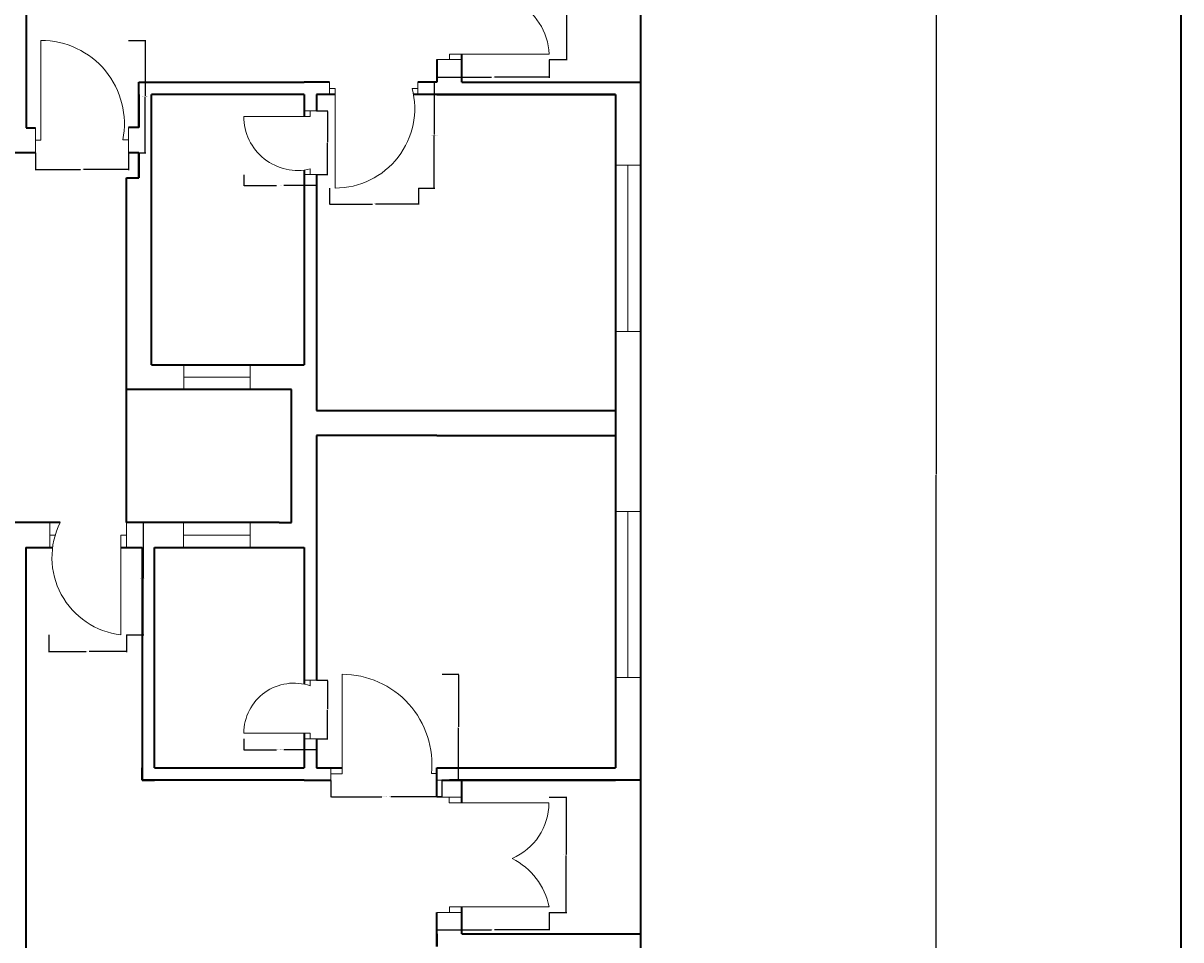
# Model space of a CAD drawing. Units: inches. Extents: x 2250 to 3629, y 982 to 2740.
# Tile 9 of 12: x 3211 to 3629, y 1497 to 1828. Entities that reach past the tile are written whole.
import ezdxf

# ---------------------------------------------------------------- set-up
doc = ezdxf.new("R2010")
doc.units = ezdxf.units.IN
for name, color, linetype, lineweight in [('A-ANNO-DIMS', 2, 'Continuous', 18), ('A-ANNO-TTLB', 7, 'Continuous', 35), ('A-DOOR', 3, 'Continuous', 18), ('A-GLAZ', 4, 'Continuous', 18), ('A-WALL', 7, 'Continuous', 35)]:
    doc.layers.add(name, color=color, linetype=linetype, lineweight=lineweight)
doc.styles.get("Standard").update_dxf_attribs({"font": 'arial.ttf'})
doc.dimstyles.get("Standard").update_dxf_attribs({"dimtxt": 0.18, "dimasz": 0.18, "dimexe": 0.18, "dimexo": 0.0625, "dimgap": 0.09, "dimtad": 0, "dimtih": 1, "dimtoh": 1, "dimdec": 4, "dimzin": 0, "dimdsep": 46, "dimtxsty": 'Standard', "dimcen": 0.09, "dimadec": 0, "dimazin": 0, "dimtfac": 1, "dimtdec": 4, "dimtofl": 0, "dimtmove": 0, "dimatfit": 3, "dimfxl": 1, "dimtolj": 1, "dimtzin": 0, "dimarcsym": 0})

# ---------------------------------------------------------------- blocks, each defined once
blk = doc.blocks.new('DR-36-BED-EAST-N')
for p, q in [((0, 38.25), (0, 33.75)), ((31.87, 33.75), (31.87, 38.25)), ((31.87, 38.25), (31.87, 36)), ((0, 33.75), (0, 36)), ((0, 36), (2, 36)), ((2, 36), (2, 0)), ((31.87, 36), (29.87, 36))]:
    blk.add_line(p, q)
blk.add_arc((2, 28.78), 28.78, 270, 14.5177)
blk = doc.blocks.new('DR-72-DECK-EAST-N')
for p, q in [((9, 42.6), (0, 42.6)), ((0, 42.6), (4.5, 42.6)), ((4.5, 42.6), (4.5, 40.6)), ((4.5, 40.6), (40.5, 40.6)), ((9, 0), (0, 0)), ((0, 0), (4.5, 0)), ((4.5, 0), (4.5, 2)), ((4.5, 2), (40.5, 2))]:
    blk.add_line(p, q)
for centre, radius, start, end in [((18.63, 40.6), 21.87, 295.9981, 0), ((18.59, 1.24), 21.93, 1.9829, 63.9515)]:
    blk.add_arc(centre, radius, start, end)
blk = doc.blocks.new('DR-36-BED-EAST-S')
for p, q in [((4, 2.25), (4, 38.25)), ((0, 4.5), (0, 0)), ((0, 0), (0, 2.25)), ((0, 2.25), (2, 2.25)), ((2, 2.25), (4, 2.25)), ((38.26, 2.37), (36.26, 2.37)), ((40.06, 0), (38.26, 0))]:
    blk.add_line(p, q)
blk.add_arc((4, 5.8), 32.45, 353.93, 90)
blk = doc.blocks.new('DR-72-DECK-EAST-S')
for p, q in [((5.33, 41.58), (0, 41.58)), ((0, 41.58), (4.45, 41.58)), ((9, 41.58), (1.67, 41.58)), ((1.67, 41.58), (5.33, 41.58)), ((4.45, 41.58), (4.45, 39.58)), ((4.45, 39.58), (40.45, 39.58)), ((4.5, 0), (4.5, 2)), ((4.5, 2), (40.5, 2)), ((9, 0), (0, 0)), ((0, 0), (4.5, 0))]:
    blk.add_line(p, q)
for centre, radius, start, end in [((18.64, 39.58), 21.82, 293.079, 0), ((16.02, -2.8), 24.94, 11.0871, 63.4091)]:
    blk.add_arc(centre, radius, start, end)
blk = doc.blocks.new('DR-24-BATH-EAST-S')
for p, q in [((21.75, 21.12), (26.25, 21.12)), ((26.25, 21.12), (24, 21.12)), ((24, 21.12), (24, 19.12)), ((24, 2), (0, 2)), ((24, 0), (24, 2)), ((26.25, 0), (21.75, 0)), ((21.75, 0), (24, 0))]:
    blk.add_line(p, q)
blk.add_arc((18.1, 2), 18.1, 70.988, 180)
blk = doc.blocks.new('DR-36-ENTRY-SE')
for p, q in [((0, 31.5), (0, 40.5)), ((27.72, 40.5), (27.72, 31.5)), ((0, 36), (2, 36)), ((27.72, 36), (25.72, 36)), ((25.72, 36), (25.72, 0)), ((27.72, 31.5), (27.72, 36))]:
    blk.add_line(p, q)
blk.add_arc((28.88, 27.9), 28.08, 153.3297, 263.5366)
blk = doc.blocks.new('DR-24-BATH-EAST-N')
for p, q in [((24, 20.95), (0, 20.95)), ((26.25, 22.95), (21.75, 22.95)), ((21.75, 22.95), (24, 22.95)), ((24, 22.95), (24, 20.95)), ((24, 0), (24, 2)), ((21.75, 0), (26.25, 0)), ((26.25, 0), (24, 0))]:
    blk.add_line(p, q)
blk.add_arc((19.48, 20.95), 19.48, 180, 283.4076)
blk = doc.blocks.new('DR-36-ENTRY-NE')
for p, q in [((2, 4.58), (2, 40.58)), ((0, 9), (0, 0)), ((33.56, 9.15), (33.56, 0.15)), ((0, 4.58), (2, 4.58)), ((33.56, 4.65), (31.56, 4.65))]:
    blk.add_line(p, q)
blk.add_arc((2, 10.45), 30.13, 348.9073, 90)
blk = doc.blocks.new('WIN-24-BATH-NW')
for p, q in [((9, 24), (0, 24)), ((0, 24), (4.5, 24)), ((4.5, 24), (4.5, 0)), ((9, 0), (0, 0)), ((4.5, 0), (9, 0))]:
    blk.add_line(p, q)
blk = doc.blocks.new('WIN-60-BED-EAST-S')
for p, q in [((0, 60), (9, 60)), ((9, 60), (4.5, 60)), ((4.5, 60), (4.5, 0)), ((9, 0), (0, 0)), ((4.5, 0), (9, 0))]:
    blk.add_line(p, q)
blk = doc.blocks.new('*D113')
at = {"layer": 'A-ANNO-DIMS', "color": 0, "lineweight": -2, "transparency": 16777216}
for p, q in [((3354.1, 1806.24), (3359.95, 1806.24)), ((3359.77, 1806.06), (3359.77, 1787.29)), ((3359.77, 1768.17), (3359.77, 1786.93)), ((3354.1, 1767.99), (3359.95, 1767.99))]:
    blk.add_line(p, q, dxfattribs=at)
at = {"layer": 'A-ANNO-DIMS', "color": 0, "transparency": 16777216}
for points in [[(3359.74, 1806.06), (3359.8, 1806.06), (3359.77, 1806.24)], [(3359.74, 1768.17), (3359.8, 1768.17), (3359.77, 1767.99)]]:
    blk.add_solid(points, dxfattribs=at)
at = {"layer": 'Defpoints', "color": 0, "transparency": 16777216}
for p in [(3354.04, 1806.24), (3359.77, 1806.24), (3354.04, 1767.99)]:
    blk.add_point(p, dxfattribs=at)
at = {"layer": 'A-ANNO-DIMS', "color": 0, "transparency": 16777216, "insert": (3359.77, 1787.11), "char_height": 0.18, "attachment_point": 5}
blk.add_mtext('\\A1;BEDROOM DOOR 38 TYP.', dxfattribs=at)
blk = doc.blocks.new('*D114')
at = {"layer": 'A-ANNO-DIMS', "color": 0, "lineweight": -2, "transparency": 16777216}
for p, q in [((3321.94, 1767.92), (3321.94, 1762.07)), ((3354.04, 1767.92), (3354.04, 1762.07)), ((3322.12, 1762.25), (3337.46, 1762.25)), ((3353.86, 1762.25), (3338.52, 1762.25))]:
    blk.add_line(p, q, dxfattribs=at)
at = {"layer": 'A-ANNO-DIMS', "color": 0, "transparency": 16777216}
for points in [[(3322.12, 1762.28), (3322.12, 1762.22), (3321.94, 1762.25)], [(3353.86, 1762.28), (3353.86, 1762.22), (3354.04, 1762.25)]]:
    blk.add_solid(points, dxfattribs=at)
at = {"layer": 'Defpoints', "color": 0, "transparency": 16777216}
for p in [(3321.94, 1767.99), (3354.04, 1767.99), (3354.04, 1762.25)]:
    blk.add_point(p, dxfattribs=at)
at = {"layer": 'A-ANNO-DIMS', "color": 0, "transparency": 16777216, "insert": (3337.99, 1762.25), "char_height": 0.18, "attachment_point": 5}
blk.add_mtext('\\A1;32 TYP.', dxfattribs=at)
blk = doc.blocks.new('*D115')
at = {"layer": 'A-ANNO-DIMS', "color": 0, "lineweight": -2, "transparency": 16777216}
for p, q in [((3401.29, 1856.98), (3407.8, 1856.98)), ((3407.62, 1856.8), (3407.62, 1835.86)), ((3407.62, 1814.56), (3407.62, 1835.5)), ((3401.29, 1814.38), (3407.8, 1814.38))]:
    blk.add_line(p, q, dxfattribs=at)
at = {"layer": 'A-ANNO-DIMS', "color": 0, "transparency": 16777216}
for points in [[(3407.59, 1856.8), (3407.65, 1856.8), (3407.62, 1856.98)], [(3407.59, 1814.56), (3407.65, 1814.56), (3407.62, 1814.38)]]:
    blk.add_solid(points, dxfattribs=at)
at = {"layer": 'Defpoints', "color": 0, "transparency": 16777216}
for p in [(3401.23, 1856.98), (3407.62, 1856.98), (3401.23, 1814.38)]:
    blk.add_point(p, dxfattribs=at)
at = {"layer": 'A-ANNO-DIMS', "color": 0, "transparency": 16777216, "insert": (3407.62, 1835.68), "char_height": 0.18, "attachment_point": 5}
blk.add_mtext('\\A1;DECK DOOR 43 TYP.', dxfattribs=at)
blk = doc.blocks.new('*D116')
at = {"layer": 'A-ANNO-DIMS', "color": 0, "lineweight": -2, "transparency": 16777216}
for p, q in [((3360.73, 1814.32), (3360.73, 1807.81)), ((3401.23, 1814.32), (3401.23, 1807.81)), ((3360.91, 1807.99), (3380.45, 1807.99)), ((3401.05, 1807.99), (3381.51, 1807.99))]:
    blk.add_line(p, q, dxfattribs=at)
at = {"layer": 'A-ANNO-DIMS', "color": 0, "transparency": 16777216}
for points in [[(3360.91, 1808.02), (3360.91, 1807.96), (3360.73, 1807.99)], [(3401.05, 1808.02), (3401.05, 1807.96), (3401.23, 1807.99)]]:
    blk.add_solid(points, dxfattribs=at)
at = {"layer": 'Defpoints', "color": 0, "transparency": 16777216}
for p in [(3360.73, 1814.38), (3401.23, 1814.38), (3401.23, 1807.99)]:
    blk.add_point(p, dxfattribs=at)
at = {"layer": 'A-ANNO-DIMS', "color": 0, "transparency": 16777216, "insert": (3380.98, 1807.99), "char_height": 0.18, "attachment_point": 5}
blk.add_mtext('\\A1;41 TYP.', dxfattribs=at)
blk = doc.blocks.new('*D117')
at = {"layer": 'A-ANNO-DIMS', "color": 0, "lineweight": -2, "transparency": 16777216}
for p, q in [((3322.46, 1554.17), (3322.46, 1548.05)), ((3362.53, 1554.17), (3362.53, 1548.05)), ((3322.64, 1548.23), (3340.87, 1548.23)), ((3362.35, 1548.23), (3344.11, 1548.23))]:
    blk.add_line(p, q, dxfattribs=at)
at = {"layer": 'A-ANNO-DIMS', "color": 0, "transparency": 16777216}
for points in [[(3322.64, 1548.26), (3322.64, 1548.2), (3322.46, 1548.23)], [(3362.35, 1548.26), (3362.35, 1548.2), (3362.53, 1548.23)]]:
    blk.add_solid(points, dxfattribs=at)
at = {"layer": 'Defpoints', "color": 0, "transparency": 16777216}
for p in [(3322.46, 1554.24), (3362.53, 1554.24), (3362.53, 1548.23)]:
    blk.add_point(p, dxfattribs=at)
at = {"layer": 'A-ANNO-DIMS', "color": 0, "transparency": 16777216, "insert": (3342.49, 1548.23), "char_height": 0.18, "attachment_point": 5}
blk.add_mtext('\\A1;BEDROOM DOOR 40 TYP.', dxfattribs=at)
blk = doc.blocks.new('*D118')
at = {"layer": 'A-ANNO-DIMS', "color": 0, "lineweight": -2, "transparency": 16777216}
for p, q in [((3362.59, 1592.49), (3368.71, 1592.49)), ((3368.53, 1592.31), (3368.53, 1573.54)), ((3368.53, 1554.42), (3368.53, 1573.18)), ((3362.59, 1554.24), (3368.71, 1554.24))]:
    blk.add_line(p, q, dxfattribs=at)
at = {"layer": 'A-ANNO-DIMS', "color": 0, "transparency": 16777216}
for points in [[(3368.5, 1592.31), (3368.56, 1592.31), (3368.53, 1592.49)], [(3368.5, 1554.42), (3368.56, 1554.42), (3368.53, 1554.24)]]:
    blk.add_solid(points, dxfattribs=at)
at = {"layer": 'Defpoints', "color": 0, "transparency": 16777216}
for p in [(3362.53, 1592.49), (3368.53, 1592.49), (3362.53, 1554.24)]:
    blk.add_point(p, dxfattribs=at)
at = {"layer": 'A-ANNO-DIMS', "color": 0, "transparency": 16777216, "insert": (3368.53, 1573.36), "char_height": 0.18, "attachment_point": 5}
blk.add_mtext('\\A1;38 TYP.', dxfattribs=at)
blk = doc.blocks.new('*D119')
at = {"layer": 'A-ANNO-DIMS', "color": 0, "lineweight": -2, "transparency": 16777216}
for p, q in [((3401.29, 1548.06), (3407.64, 1548.06)), ((3407.46, 1547.88), (3407.46, 1527.45)), ((3407.46, 1506.66), (3407.46, 1527.09)), ((3401.29, 1506.48), (3407.64, 1506.48))]:
    blk.add_line(p, q, dxfattribs=at)
at = {"layer": 'A-ANNO-DIMS', "color": 0, "transparency": 16777216}
for points in [[(3407.43, 1547.88), (3407.49, 1547.88), (3407.46, 1548.06)], [(3407.43, 1506.66), (3407.49, 1506.66), (3407.46, 1506.48)]]:
    blk.add_solid(points, dxfattribs=at)
at = {"layer": 'Defpoints', "color": 0, "transparency": 16777216}
for p in [(3401.23, 1548.06), (3407.46, 1548.06), (3401.23, 1506.48)]:
    blk.add_point(p, dxfattribs=at)
at = {"layer": 'A-ANNO-DIMS', "color": 0, "transparency": 16777216, "insert": (3407.46, 1527.27), "char_height": 0.18, "attachment_point": 5}
blk.add_mtext('\\A1;DECK DOOR 42 TYP.', dxfattribs=at)
blk = doc.blocks.new('*D120')
at = {"layer": 'A-ANNO-DIMS', "color": 0, "lineweight": -2, "transparency": 16777216}
for p, q in [((3360.73, 1506.42), (3360.73, 1500.06)), ((3401.23, 1506.42), (3401.23, 1500.06)), ((3360.91, 1500.24), (3380.45, 1500.24)), ((3401.05, 1500.24), (3381.51, 1500.24))]:
    blk.add_line(p, q, dxfattribs=at)
at = {"layer": 'A-ANNO-DIMS', "color": 0, "transparency": 16777216}
for points in [[(3360.91, 1500.27), (3360.91, 1500.21), (3360.73, 1500.24)], [(3401.05, 1500.27), (3401.05, 1500.21), (3401.23, 1500.24)]]:
    blk.add_solid(points, dxfattribs=at)
at = {"layer": 'Defpoints', "color": 0, "transparency": 16777216}
for p in [(3360.73, 1506.48), (3401.23, 1506.48), (3401.23, 1500.24)]:
    blk.add_point(p, dxfattribs=at)
at = {"layer": 'A-ANNO-DIMS', "color": 0, "transparency": 16777216, "insert": (3380.98, 1500.24), "char_height": 0.18, "attachment_point": 5}
blk.add_mtext('\\A1;41 TYP.', dxfattribs=at)
blk = doc.blocks.new('*D131')
at = {"layer": 'A-ANNO-DIMS', "color": 0, "lineweight": -2, "transparency": 16777216}
for p, q in [((3290.98, 1569.11), (3290.98, 1565.05)), ((3317.23, 1569.11), (3317.23, 1565.05)), ((3291.16, 1565.23), (3302.8, 1565.23)), ((3317.05, 1565.23), (3305.41, 1565.23))]:
    blk.add_line(p, q, dxfattribs=at)
at = {"layer": 'A-ANNO-DIMS', "color": 0, "transparency": 16777216}
for points in [[(3291.16, 1565.26), (3291.16, 1565.2), (3290.98, 1565.23)], [(3317.05, 1565.26), (3317.05, 1565.2), (3317.23, 1565.23)]]:
    blk.add_solid(points, dxfattribs=at)
at = {"layer": 'Defpoints', "color": 0, "transparency": 16777216}
for p in [(3290.98, 1569.17), (3317.23, 1569.17), (3317.23, 1565.23)]:
    blk.add_point(p, dxfattribs=at)
at = {"layer": 'A-ANNO-DIMS', "color": 0, "transparency": 16777216, "insert": (3304.1, 1565.23), "char_height": 0.18, "attachment_point": 5}
blk.add_mtext('\\A1;BATH DOOR 26 TYP.', dxfattribs=at)
blk = doc.blocks.new('*D132')
at = {"layer": 'A-ANNO-DIMS', "color": 0, "lineweight": -2, "transparency": 16777216}
for p, q in [((3317.29, 1590.29), (3321.34, 1590.29)), ((3321.16, 1590.11), (3321.16, 1579.91)), ((3321.16, 1569.35), (3321.16, 1579.55)), ((3317.29, 1569.17), (3321.34, 1569.17))]:
    blk.add_line(p, q, dxfattribs=at)
at = {"layer": 'A-ANNO-DIMS', "color": 0, "transparency": 16777216}
for points in [[(3321.13, 1590.11), (3321.19, 1590.11), (3321.16, 1590.29)], [(3321.13, 1569.35), (3321.19, 1569.35), (3321.16, 1569.17)]]:
    blk.add_solid(points, dxfattribs=at)
at = {"layer": 'Defpoints', "color": 0, "transparency": 16777216}
for p in [(3317.23, 1590.29), (3321.16, 1590.29), (3317.23, 1569.17)]:
    blk.add_point(p, dxfattribs=at)
at = {"layer": 'A-ANNO-DIMS', "color": 0, "transparency": 16777216, "insert": (3321.16, 1579.73), "char_height": 0.18, "attachment_point": 5}
blk.add_mtext('\\A1;21 TYP.', dxfattribs=at)
blk = doc.blocks.new('*D133')
at = {"layer": 'A-ANNO-DIMS', "color": 0, "lineweight": -2, "transparency": 16777216}
for p, q in [((3248.66, 1647.24), (3254.85, 1647.24)), ((3254.67, 1647.06), (3254.67, 1627.17)), ((3254.67, 1606.92), (3254.67, 1626.8)), ((3248.66, 1606.74), (3254.85, 1606.74))]:
    blk.add_line(p, q, dxfattribs=at)
at = {"layer": 'A-ANNO-DIMS', "color": 0, "transparency": 16777216}
for points in [[(3254.64, 1647.06), (3254.7, 1647.06), (3254.67, 1647.24)], [(3254.64, 1606.92), (3254.7, 1606.92), (3254.67, 1606.74)]]:
    blk.add_solid(points, dxfattribs=at)
at = {"layer": 'Defpoints', "color": 0, "transparency": 16777216}
for p in [(3248.6, 1647.24), (3254.67, 1647.24), (3248.6, 1606.74)]:
    blk.add_point(p, dxfattribs=at)
at = {"layer": 'A-ANNO-DIMS', "color": 0, "transparency": 16777216, "insert": (3254.67, 1626.99), "char_height": 0.18, "attachment_point": 5}
blk.add_mtext('\\A1;ENTRY DOOR 41 TYP.', dxfattribs=at)
blk = doc.blocks.new('*D134')
at = {"layer": 'A-ANNO-DIMS', "color": 0, "lineweight": -2, "transparency": 16777216}
for p, q in [((3220.55, 1606.67), (3220.55, 1600.48)), ((3248.6, 1606.67), (3248.6, 1600.48)), ((3220.73, 1600.66), (3234.04, 1600.66)), ((3248.42, 1600.66), (3235.1, 1600.66))]:
    blk.add_line(p, q, dxfattribs=at)
at = {"layer": 'A-ANNO-DIMS', "color": 0, "transparency": 16777216}
for points in [[(3220.73, 1600.69), (3220.73, 1600.63), (3220.55, 1600.66)], [(3248.42, 1600.69), (3248.42, 1600.63), (3248.6, 1600.66)]]:
    blk.add_solid(points, dxfattribs=at)
at = {"layer": 'Defpoints', "color": 0, "transparency": 16777216}
for p in [(3220.55, 1606.74), (3248.6, 1606.74), (3248.6, 1600.66)]:
    blk.add_point(p, dxfattribs=at)
at = {"layer": 'A-ANNO-DIMS', "color": 0, "transparency": 16777216, "insert": (3234.57, 1600.66), "char_height": 0.18, "attachment_point": 5}
blk.add_mtext('\\A1;28 TYP.', dxfattribs=at)
blk = doc.blocks.new('*D139')
at = {"layer": 'A-ANNO-DIMS', "color": 0, "lineweight": -2, "transparency": 16777216}
for p, q in [((3290.98, 1772.83), (3290.98, 1768.77)), ((3291.16, 1768.95), (3302.8, 1768.95)), ((3317.05, 1768.95), (3305.41, 1768.95)), ((3317.23, 1772.83), (3317.23, 1768.77))]:
    blk.add_line(p, q, dxfattribs=at)
at = {"layer": 'A-ANNO-DIMS', "color": 0, "transparency": 16777216}
for points in [[(3291.16, 1768.98), (3291.16, 1768.92), (3290.98, 1768.95)], [(3317.05, 1768.98), (3317.05, 1768.92), (3317.23, 1768.95)]]:
    blk.add_solid(points, dxfattribs=at)
at = {"layer": 'Defpoints', "color": 0, "transparency": 16777216}
for p in [(3290.98, 1772.89), (3317.23, 1772.89), (3317.23, 1768.95)]:
    blk.add_point(p, dxfattribs=at)
at = {"layer": 'A-ANNO-DIMS', "color": 0, "transparency": 16777216, "insert": (3304.1, 1768.95), "char_height": 0.18, "attachment_point": 5}
blk.add_mtext('\\A1;BATH DOOR 26 TYP.', dxfattribs=at)
blk = doc.blocks.new('*D140')
at = {"layer": 'A-ANNO-DIMS', "color": 0, "lineweight": -2, "transparency": 16777216}
for p, q in [((3317.29, 1795.84), (3321.34, 1795.84)), ((3321.16, 1795.66), (3321.16, 1784.55)), ((3321.16, 1773.07), (3321.16, 1784.18)), ((3317.29, 1772.89), (3321.34, 1772.89))]:
    blk.add_line(p, q, dxfattribs=at)
at = {"layer": 'A-ANNO-DIMS', "color": 0, "transparency": 16777216}
for points in [[(3321.13, 1795.66), (3321.19, 1795.66), (3321.16, 1795.84)], [(3321.13, 1773.07), (3321.19, 1773.07), (3321.16, 1772.89)]]:
    blk.add_solid(points, dxfattribs=at)
at = {"layer": 'Defpoints', "color": 0, "transparency": 16777216}
for p in [(3317.23, 1795.84), (3321.16, 1795.84), (3317.23, 1772.89)]:
    blk.add_point(p, dxfattribs=at)
at = {"layer": 'A-ANNO-DIMS', "color": 0, "transparency": 16777216, "insert": (3321.16, 1784.37), "char_height": 0.18, "attachment_point": 5}
blk.add_mtext('\\A1;23 TYP.', dxfattribs=at)
blk = doc.blocks.new('*D145')
at = {"layer": 'A-ANNO-DIMS', "color": 0, "lineweight": -2, "transparency": 16777216}
for p, q in [((3249.35, 1821.31), (3255.55, 1821.31)), ((3255.37, 1821.13), (3255.37, 1801.21)), ((3255.37, 1780.92), (3255.37, 1800.84)), ((3249.35, 1780.74), (3255.55, 1780.74))]:
    blk.add_line(p, q, dxfattribs=at)
at = {"layer": 'A-ANNO-DIMS', "color": 0, "transparency": 16777216}
for points in [[(3255.34, 1821.13), (3255.4, 1821.13), (3255.37, 1821.31)], [(3255.34, 1780.92), (3255.4, 1780.92), (3255.37, 1780.74)]]:
    blk.add_solid(points, dxfattribs=at)
at = {"layer": 'Defpoints', "color": 0, "transparency": 16777216}
for p in [(3249.29, 1821.31), (3255.37, 1821.31), (3249.29, 1780.74)]:
    blk.add_point(p, dxfattribs=at)
at = {"layer": 'A-ANNO-DIMS', "color": 0, "transparency": 16777216, "insert": (3255.37, 1801.02), "char_height": 0.18, "attachment_point": 5}
blk.add_mtext('\\A1;ENTRY DOOR 41 TYP.', dxfattribs=at)
blk = doc.blocks.new('*D146')
at = {"layer": 'A-ANNO-DIMS', "color": 0, "lineweight": -2, "transparency": 16777216}
for p, q in [((3215.72, 1780.67), (3215.72, 1774.47)), ((3249.29, 1780.67), (3249.29, 1774.47)), ((3215.9, 1774.65), (3231.97, 1774.65)), ((3249.11, 1774.65), (3233.03, 1774.65))]:
    blk.add_line(p, q, dxfattribs=at)
at = {"layer": 'A-ANNO-DIMS', "color": 0, "transparency": 16777216}
for points in [[(3215.9, 1774.68), (3215.9, 1774.62), (3215.72, 1774.65)], [(3249.11, 1774.68), (3249.11, 1774.62), (3249.29, 1774.65)]]:
    blk.add_solid(points, dxfattribs=at)
at = {"layer": 'Defpoints', "color": 0, "transparency": 16777216}
for p in [(3215.72, 1780.74), (3249.29, 1780.74), (3249.29, 1774.65)]:
    blk.add_point(p, dxfattribs=at)
at = {"layer": 'A-ANNO-DIMS', "color": 0, "transparency": 16777216, "insert": (3232.5, 1774.65), "char_height": 0.18, "attachment_point": 5}
blk.add_mtext('\\A1;34 TYP.', dxfattribs=at)
blk = doc.blocks.new('*D172')
at = {"layer": 'A-ANNO-DIMS', "color": 0, "lineweight": -2, "transparency": 16777216}
for p, q in [((3433.02, 2070.24), (3541.21, 2070.24)), ((3541.03, 2070.06), (3541.03, 1664.67)), ((3541.03, 1258.92), (3541.03, 1664.3)), ((3059.29, 1258.74), (3541.21, 1258.74))]:
    blk.add_line(p, q, dxfattribs=at)
at = {"layer": 'A-ANNO-DIMS', "color": 0, "transparency": 16777216}
for points in [[(3541, 2070.06), (3541.06, 2070.06), (3541.03, 2070.24)], [(3541, 1258.92), (3541.06, 1258.92), (3541.03, 1258.74)]]:
    blk.add_solid(points, dxfattribs=at)
at = {"layer": 'Defpoints', "color": 0, "transparency": 16777216}
for p in [(3432.96, 2070.24), (3541.03, 2070.24), (3059.23, 1258.74)]:
    blk.add_point(p, dxfattribs=at)
at = {"layer": 'A-ANNO-DIMS', "color": 0, "transparency": 16777216, "insert": (3541.03, 1664.49), "char_height": 0.18, "attachment_point": 5}
blk.add_mtext('\\A1;811.5', dxfattribs=at)

msp = doc.modelspace()

# ---------------------------------------------------------------- linework, layer by layer
at = {"layer": 'A-ANNO-TTLB'}
msp.add_lwpolyline([(2249.6849, 2739.593), (3629.4532, 2739.593), (3629.4532, 982.3108), (2249.6849, 982.3108)], close=True, dxfattribs=at)
at = {"layer": 'A-WALL'}
for p, q in [((3434.2267, 2029.7354), (3434.2267, 1276.7354)), ((3212.321, 1926.2354), (3212.321, 1789.7354)), ((3369.7267, 1806.2354), (3369.7267, 1816.3801)), ((3360.7267, 1814.3801), (3360.7267, 1806.2354)), ((3253.0965, 1806.2354), (3312.7267, 1806.2354)), ((3253.0965, 1789.8862), (3253.0965, 1806.2354)), ((3321.9387, 1806.2354), (3312.7267, 1806.2354)), ((3360.7267, 1806.2354), (3353.804, 1806.2354)), ((3369.7267, 1806.2354), (3434.2267, 1806.2354)), ((3253.0965, 1801.7354), (3253.0965, 1789.8862)), ((3312.7267, 1801.7354), (3257.5965, 1801.7354)), ((3257.5965, 1704.2354), (3257.5965, 1801.7354)), ((3312.7267, 1801.7354), (3312.7267, 1793.8422)), ((3323.9387, 1801.7354), (3317.2267, 1801.7354)), ((3317.2267, 1801.7354), (3317.2267, 1795.8422)), ((3425.2267, 1801.7354), (3352.2915, 1801.7354)), ((3360.7267, 1801.7354), (3425.2267, 1801.7354)), ((3360.7267, 1801.7354), (3369.7267, 1801.7354)), ((3425.2267, 1801.7354), (3425.2267, 1558.7354)), ((3253.0965, 1789.8862), (3249.2854, 1789.8862)), ((3212.321, 1789.7354), (3215.7202, 1789.7354)), ((3212.321, 1780.7354), (3203.2267, 1780.7354)), ((3215.7202, 1780.7354), (3212.321, 1780.7354)), ((3249.2854, 1780.8862), (3253.0965, 1780.8862)), ((3253.0965, 1780.8862), (3253.0965, 1771.6808)), ((3253.0965, 1771.6808), (3253.0965, 1780.8862)), ((3312.7267, 1774.4922), (3312.7267, 1704.2354)), ((3248.5965, 1704.2354), (3248.5965, 1771.6808)), ((3248.5965, 1771.6808), (3253.0965, 1771.6808)), ((3317.2267, 1772.8908), (3317.2267, 1687.7354)), ((3248.5965, 1647.2354), (3248.5965, 1704.2354)), ((3257.5965, 1704.2354), (3312.7267, 1704.2354)), ((3308.2267, 1695.2354), (3248.5965, 1695.2354)), ((3308.2267, 1647.2354), (3308.2267, 1695.2354)), ((3317.2267, 1687.7354), (3360.7267, 1687.7354)), ((3360.7267, 1687.7354), (3425.2267, 1687.7354)), ((3360.7267, 1678.7354), (3317.2267, 1678.7354)), ((3317.2267, 1678.7354), (3317.2267, 1590.2852)), ((3360.7267, 1678.7354), (3425.2267, 1678.7354)), ((3224.6679, 1647.2354), (3200.6151, 1647.2354)), ((3254.2267, 1647.2354), (3248.5965, 1647.2354)), ((3303.7267, 1647.2354), (3254.2267, 1647.2354)), ((3303.7267, 1647.2354), (3308.2267, 1647.2354)), ((3212.2267, 1638.2354), (3212.2267, 1434.2354)), ((3212.2267, 1638.2354), (3221.9128, 1638.2354)), ((3246.5965, 1638.2354), (3254.2267, 1638.2354)), ((3254.2267, 1638.2354), (3254.2267, 1554.2354)), ((3258.7267, 1558.7354), (3258.7267, 1638.2354)), ((3258.7267, 1638.2354), (3312.7267, 1638.2354)), ((3312.7267, 1638.2354), (3312.7267, 1588.9015)), ((3312.7267, 1638.2354), (3312.7267, 1588.9015)), ((3312.7267, 1571.1699), (3312.7267, 1558.7354)), ((3312.7267, 1571.1699), (3312.7267, 1558.7354)), ((3317.2267, 1569.1699), (3317.2267, 1558.7354)), ((3254.2267, 1554.2354), (3254.2267, 1558.7354)), ((3258.7267, 1558.7354), (3312.7267, 1558.7354)), ((3317.2267, 1558.7354), (3326.4621, 1558.7354)), ((3360.7267, 1558.7354), (3425.2267, 1558.7354)), ((3360.7267, 1548.0588), (3360.7267, 1558.7354)), ((3254.2267, 1554.2354), (3258.7267, 1554.2354)), ((3258.7267, 1554.2354), (3254.2267, 1554.2354)), ((3312.7267, 1554.2354), (3258.7267, 1554.2354)), ((3312.7267, 1554.2354), (3322.4621, 1554.2354)), ((3362.5252, 1554.2354), (3425.2267, 1554.2354)), ((3434.2267, 1554.2354), (3365.2267, 1554.2354)), ((3369.7267, 1546.0588), (3369.7267, 1554.2354)), ((3360.7267, 1494.2354), (3360.7267, 1506.4808)), ((3369.7267, 1498.7354), (3369.7267, 1508.4808)), ((3360.7267, 1498.7354), (3360.7267, 1494.2354)), ((3369.7267, 1498.7354), (3434.2267, 1498.7354))]:
    msp.add_line(p, q, dxfattribs=at)

# ---------------------------------------------------------------- block references
at = {"layer": 'A-DOOR'}
for name, p in [('DR-72-DECK-EAST-N', (3360.7265, 1814.38)), ('DR-36-ENTRY-NE', (3215.7205, 1780.735)), ('DR-36-BED-EAST-N', (3321.9385, 1767.985)), ('DR-24-BATH-EAST-N', (3290.9765, 1772.891)), ('DR-36-ENTRY-SE', (3220.8755, 1606.735)), ('DR-24-BATH-EAST-S', (3290.9765, 1569.17)), ('DR-36-BED-EAST-S', (3322.4625, 1554.235)), ('DR-72-DECK-EAST-S', (3360.7265, 1506.481))]:
    msp.add_blockref(name, p, dxfattribs=at)
at = {"layer": 'A-GLAZ'}
for p in [(3425.2265, 1716.2735), (3425.2265, 1591.289)]:
    msp.add_blockref('WIN-60-BED-EAST-S', p, dxfattribs=at)
for p, rotation in [((3293.2826, 1695.2352), 89.99999999999737), ((3293.237, 1638.2448), 90.04567875527518)]:
    msp.add_blockref('WIN-24-BATH-NW', p, dxfattribs=dict(at, rotation=rotation))

# ---------------------------------------------------------------- dimensions: what is measured, and where the dimension line sits
at = {"layer": 'A-ANNO-DIMS'}
dim = msp.add_linear_dim(base=(3541.0278, 2070.2354), p1=(3059.2267, 1258.7354), p2=(3432.9579, 2070.2354), angle=90, dimstyle='Standard', override={"dimdec": 1, "dimlfac": 1, "dimrnd": 0, "dimzin": 0, "dimdsep": 46, "dimlunit": 2}, dxfattribs=at)
dim.commit()
dim.dimension.update_dxf_attribs({"geometry": '*D172', "text_midpoint": (3541.0278, 1664.4854)})
for base, p1, p2, text, picture, middle in [((3407.6165, 1856.9787), (3401.2267, 1814.3801), (3401.2267, 1856.9787), 'DECK DOOR <> TYP.', '*D115', (3407.6165, 1835.6794)), ((3255.3717, 1821.3108), (3249.2854, 1780.7354), (3249.2854, 1821.3108), 'ENTRY DOOR <> TYP.', '*D145', (3255.3717, 1801.0231)), ((3359.7741, 1806.2354), (3354.0366, 1767.9854), (3354.0366, 1806.2354), 'BEDROOM DOOR <> TYP.', '*D113', (3359.7741, 1787.1104)), ((3321.1642, 1795.8422), (3317.2267, 1772.8908), (3317.2267, 1795.8422), '<> TYP.', '*D140', (3321.1642, 1784.3665)), ((3254.6714617036, 1647.2354249075), (3248.5964617036, 1606.7354249075), (3248.5964617036, 1647.2354249075), 'ENTRY DOOR <> TYP.', '*D133', (3254.6714617036, 1626.9854249075)), ((3321.1642, 1590.2852), (3317.2267, 1569.1699), (3317.2267, 1590.2852), '<> TYP.', '*D132', (3321.1642, 1579.7276)), ((3368.5347, 1592.4854), (3362.5252, 1554.2354), (3362.5252, 1592.4854), '<> TYP.', '*D118', (3368.5347, 1573.3604)), ((3407.4634, 1548.0588), (3401.2267, 1506.4808), (3401.2267, 1548.0588), 'DECK DOOR <> TYP.', '*D119', (3407.4634, 1527.2698))]:
    dim = msp.add_linear_dim(base=base, p1=p1, p2=p2, angle=90, text=text, dimstyle='Standard', override={"dimdec": 0, "dimlfac": 1, "dimrnd": 0, "dimzin": 0, "dimdsep": 46, "dimlunit": 2}, dxfattribs=at)
    dim.commit()
    dim.dimension.update_dxf_attribs({"geometry": picture, "text_midpoint": middle})
for base, p1, p2, text, picture, middle in [((3401.226726419, 1807.9903644807), (3360.726726419, 1814.3801461668), (3401.226726419, 1814.3801461668), '<> TYP.', '*D116', (3380.976726419, 1807.9903644807)), ((3249.2854, 1774.6491), (3215.7202, 1780.7354), (3249.2854, 1780.7354), '<> TYP.', '*D146', (3232.5028, 1774.6491)), ((3317.2267, 1768.9533), (3290.9767, 1772.8908), (3317.2267, 1772.8908), 'BATH DOOR <> TYP.', '*D139', (3304.1017, 1768.9533)), ((3354.0366, 1762.2479), (3321.9387, 1767.9854), (3354.0366, 1767.9854), '<> TYP.', '*D114', (3337.9876, 1762.2479)), ((3248.5965, 1600.6604), (3220.5482, 1606.7354), (3248.5965, 1606.7354), '<> TYP.', '*D134', (3234.5723, 1600.6604)), ((3317.2267, 1565.2324), (3290.9767, 1569.1699), (3317.2267, 1569.1699), 'BATH DOOR <> TYP.', '*D131', (3304.1017, 1565.2324)), ((3362.5252, 1548.226), (3322.4621, 1554.2354), (3362.5252, 1554.2354), 'BEDROOM DOOR <> TYP.', '*D117', (3342.4937, 1548.226)), ((3401.226726419, 1500.244057921), (3360.726726419, 1506.4807661183), (3401.226726419, 1506.4807661183), '<> TYP.', '*D120', (3380.976726419, 1500.244057921))]:
    dim = msp.add_linear_dim(base=base, p1=p1, p2=p2, text=text, dimstyle='Standard', override={"dimdec": 0, "dimlfac": 1, "dimrnd": 0, "dimzin": 0, "dimdsep": 46, "dimlunit": 2}, dxfattribs=at)
    dim.commit()
    dim.dimension.update_dxf_attribs({"geometry": picture, "text_midpoint": middle})

doc.saveas('drawing.dxf')
